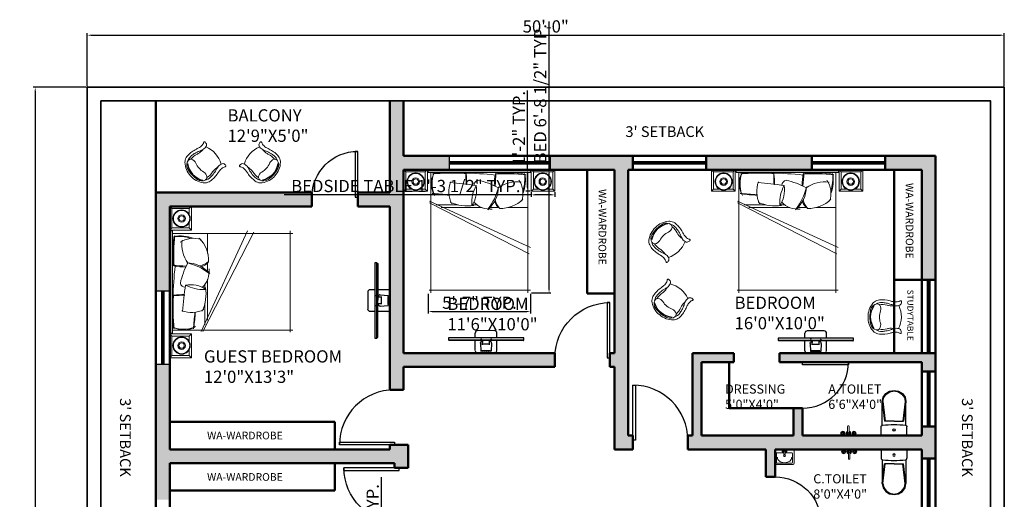
# Model space of a CAD drawing. Units: inches. Extents: x 2442 to 3851, y 589 to 2836.
# Tile 12 of 22: x 3165 to 3809, y 1732 to 2046. Entities that reach past the tile are written whole.
import ezdxf

# ---------------------------------------------------------------- set-up
doc = ezdxf.new("R2010")
doc.units = ezdxf.units.IN
for name, color, linetype, lineweight in [('0.10', 252, 'Continuous', 9), ('0.15', 34, 'Continuous', 15), ('A-ANNO-DIMS', 2, 'Continuous', 18), ('A-ANNO-TEXT', 7, 'Continuous', 18), ('A-AREA-IDEN', 7, 'Continuous', 18), ('A-DOOR', 4, 'Continuous', 25), ('A-FLOR-FIXT', 8, 'Continuous', 18), ('A-FURN', 8, 'Continuous', 18), ('A-GLAZ', 1, 'Continuous', 25), ('A-WALL', 7, 'Continuous', 50), ('A-WALL-PATT', 8, 'Continuous', 13), ('C-PROP', 7, 'Continuous', 35)]:
    doc.layers.add(name, color=color, linetype=linetype, lineweight=lineweight)
for name, color, linetype in [('IFF-FURN-DETAIL', 250, 'Continuous'), ('SANTEH', 7, 'Continuous'), ('window', 130, 'Continuous')]:
    doc.layers.add(name, color=color, linetype=linetype)
doc.styles.get("Standard").update_dxf_attribs({"font": 'arial.ttf'})
doc.dimstyles.new('ISO-25', dxfattribs={"dimtxt": 8, "dimasz": 2.5, "dimexe": 1.25, "dimexo": 0.625, "dimtad": 1, "dimlunit": 3, "dimtxsty": 'Standard', "dimcen": 2.5, "dimadec": 0, "dimazin": 0, "dimtfac": 1, "dimtmove": 0, "dimatfit": 3, "dimfxl": 1, "dimarcsym": 0})

# ---------------------------------------------------------------- blocks, each defined once
blk = doc.blocks.new('*U23')
for p, q in [((0, 0), (0, -6)), ((36, 0), (36, -6))]:
    blk.add_line(p, q)
blk.add_lwpolyline([(0, 0), (0, 36), (1.75, 36), (1.75, 0)], close=True)
blk.add_arc((0, 0), 36, 0, 90)
blk = doc.blocks.new('*U24')
for p, q in [((0, 0), (0, -6)), ((30, 0), (30, -6))]:
    blk.add_line(p, q)
blk.add_lwpolyline([(0, 0), (0, 30), (1.75, 30), (1.75, 0)], close=True)
blk.add_arc((0, 0), 30, 0, 90)
blk = doc.blocks.new('camita')
at = {"layer": '0.10'}
for p, q in [((-0.85, -0.045), (0.85, -0.045)), ((-0.805, -0.045), (-0.805, -2.048)), ((0.805, -0.045), (0.805, -2.048)), ((-0.827, -0.521), (0.846, -1.293)), ((-0.827, -0.548), (0.824, -1.399)), ((-0.716, -0.585), (-0.355, -0.585)), ((-0.638, -0.63), (0.043, -0.63)), ((-0.114, -0.585), (-0.049, -0.585)), ((0.175, -0.63), (0.318, -0.63)), ((0.474, -0.63), (0.805, -0.63)), ((-0.835, -2), (0.846, -2))]:
    blk.add_line(p, q, dxfattribs=at)
blk.add_lwpolyline([(-0.85, -0.041), (0.85, -0.041), (0.85, 0), (-0.85, 0)], close=True, dxfattribs=at)
for centre, radius, start, end in [((-0.457, -0.236), 0.344, 147.51, 213.8336), ((-0.2, -0.227), 0.586, 163.9263, 197.1409), ((-0.364, -5.846), 5.791, 83.8073, 94.1211), ((-0.51, -1.723), 1.678, 80.1255, 98.6619), ((2.353, -0.053), 2.58, 180.1063, 184.3854), ((-1.544, -0.245), 1.333, 359.9394, 7.5533), ((1.581, -0.289), 1.335, 170.3802, 178.9914), ((-1.44, -0.061), 1.712, 352.9291, 0.3959), ((0.452, -3.067), 3, 83.9026, 93.6759), ((0.486, -1.629), 1.578, 80.1602, 98.06), ((0.029, -0.138), 0.726, 342.5841, 6.0048), ((0.133, -0.17), 0.631, 339.923, 8.7433), ((-0.054, -0.363), 0.454, 159.3026, 206.5026), ((-1.33, -9.675), 9.499, 82.2708, 84.9399), ((0.458, -0.545), 0.584, 151.0456, 184.1497), ((-0.534, -0.339), 0.487, 327.2644, 9.0473), ((-0.007, -0.258), 0.0828, 100.018, 179.736), ((-0.293, -1.438), 1.29, 61.9749, 77.8435), ((-0.199, -0.274), 0.516, 310.7395, 359.0576), ((-0.567, -0.087), 0.906, 321.6953, 346.4626), ((0.627, -0.752), 0.551, 82.9691, 124.6739), ((0.32, -0.394), 0.404, 341.4524, 33.4512), ((-1.867, -14.986), 14.632, 84.6597, 85.7516), ((-0.46, 1.486), 1.909, 260.953, 268.6517), ((-0.2, 0.064), 0.667, 244.7809, 279.0606), ((0.179, -0.272), 0.383, 224.5284, 275.2229), ((0.438, -0.483), 0.19, 193.6849, 236.7035), ((0.571, -0.432), 0.315, 192.9388, 221.9636), ((0.361, -0.133), 0.51, 267.2589, 315.2997)]:
    blk.add_arc(centre, radius, start, end, dxfattribs=at)
blk = doc.blocks.new('VELADOR')
at = {"layer": '0.15'}
for p, q in [((-0.248, 0), (-0.203, -0.045)), ((0.248, 0), (0.202, -0.045)), ((-0.203, -0.405), (-0.248, -0.45)), ((0.248, -0.45), (0.202, -0.405))]:
    blk.add_line(p, q, dxfattribs=at)
blk.add_lwpolyline([(-0.248, 0), (-0.248, -0.45), (0.248, -0.45), (0.248, 0)], close=True, dxfattribs=at)
blk.add_lwpolyline([(0.092, -0.405), (0.202, -0.405), (0.202, -0.045), (-0.203, -0.045), (-0.203, -0.405), (-0.082, -0.405)], dxfattribs=at)
for radius in [0.18, 0.169, 0.0788, 0.0563]:
    blk.add_circle((0.005, -0.247), radius, dxfattribs=at)
blk = doc.blocks.new('ILNG95')
for points in [[(120, 308, -0.32971), (51, 384, -0.036099), (50, 422, -0.497733), (75, 439, -0.070621), (96, 429, 0.101868), (133, 414, 0.091794), (259, 412, 0.024114), (351, 433, -0.090294), (638, 458, -0.132412), (775, 407, -0.068618), (816, 368, -0.184346), (943, 0, 1.803905)], [(120, 308, 0.138132), (244, 313, 0.001085), (325, 339, -0.034227), (462, 375, -0.033255), (567, 387, -0.137428), (727, 350, -4.561553)], [(120, 308, 0.138132), (244, 313, 0.001085), (325, 339, -0.034227), (462, 375, -0.033255), (567, 387, -0.137428), (727, 350, -4.561553)], [(235, 308, 0.064243), (394, 307, 0.04414), (433, 315, -0.118032), (643, 329, -6.296816)], [(235, 308, 0.064243), (394, 307, 0.04414), (433, 315, -0.118032), (643, 329, -6.296816)], [(639, 0, 0.078302), (612, 161, -0.233633), (633, 315, -0.28763), (710, 349, -0.317923), (875, 193, -0.032882), (900, 0, 1.140397)], [(639, 0, 0.078302), (612, 161, -0.233633), (633, 315, -0.28763), (710, 349, -0.317923), (875, 193, -0.032882), (900, 0, 1.140397)], [(120, -308, 0.32971), (51, -384, 0.036099), (50, -422, 0.497733), (75, -439, 0.070621), (96, -429, -0.101868), (133, -414, -0.091794), (259, -412, -0.024114), (351, -433, 0.090294), (638, -458, 0.132412), (775, -407, 0.068618), (816, -368, 0.184346), (943, 0, -1.803905)], [(639, 0, -0.078302), (612, -161, 0.233633), (633, -315, 0.28763), (710, -349, 0.317923), (875, -193, 0.032882), (900, 0, -1.140397)], [(639, 0, -0.078302), (612, -161, 0.233633), (633, -315, 0.28763), (710, -349, 0.317923), (875, -193, 0.032882), (900, 0, -1.140397)], [(120, -308, -0.138132), (244, -313, -0.001085), (325, -339, 0.034227), (462, -375, 0.033255), (567, -387, 0.137428), (727, -350, 4.561553)], [(120, -308, -0.138132), (244, -313, -0.001085), (325, -339, 0.034227), (462, -375, 0.033255), (567, -387, 0.137428), (727, -350, 4.561553)], [(235, -308, -0.064243), (394, -307, -0.04414), (433, -315, 0.118032), (643, -329, 6.296816)], [(235, -308, -0.064243), (394, -307, -0.04414), (433, -315, 0.118032), (643, -329, 6.296816)]]:
    blk.add_lwpolyline(points, format="xyb")
blk.add_arc((759, 1), 709, 154.3281, 205.801)
at = {"layer": 'IFF-FURN-DETAIL'}
blk.add_arc((326, -2), 549, 326.8997, 34.6691, dxfattribs=at)
blk.add_arc((326, -2), 549, 326.8997, 34.6691, dxfattribs=at)
blk = doc.blocks.new('TV')
at = {"color": 0}
for p, q in [((3967.27, 1784.85), (3967.05, 1784.65)), ((3967.76, 1763.68), (3967.54, 1763.86))]:
    blk.add_line(p, q, dxfattribs=at)
at = {"layer": 'window'}
for p, q in [((3967.54, 1763.86), (3967.05, 1784.65)), ((3964.41, 1777.23), (3967.22, 1777.3)), ((3968.01, 1777.32), (3969.36, 1777.35)), ((3966.53, 1775.82), (3964.33, 1775.61)), ((3964.34, 1775.34), (3964.45, 1775.34)), ((3964.34, 1775.31), (3964.43, 1775.32)), ((3966.14, 1775.2), (3967.01, 1775.22)), ((3966.14, 1775.18), (3967.27, 1775.2)), ((3966.14, 1775.18), (3966.14, 1775.2)), ((3966.3, 1773.29), (3966.26, 1775.18)), ((3964.39, 1773.06), (3964.48, 1773.06)), ((3964.39, 1773.04), (3964.5, 1773.04)), ((3966.61, 1772.66), (3964.4, 1772.77)), ((3966.19, 1773.28), (3967.31, 1773.31)), ((3966.19, 1773.26), (3967.05, 1773.28)), ((3966.19, 1773.26), (3966.19, 1773.28)), ((3964.55, 1771.15), (3967.36, 1771.22)), ((3968.15, 1771.24), (3969.5, 1771.27))]:
    blk.add_line(p, q, dxfattribs=at)
for points in [[(3968.33, 1763.69), (3967.83, 1784.86), (3967.27, 1784.85), (3967.76, 1763.68), (3968.33, 1763.69)], [(3963.86, 1771.81), (3963.75, 1776.54)], [(3964.4, 1772.77), (3964.33, 1775.61)], [(3964.48, 1773.06), (3964.43, 1775.32)], [(3964.5, 1773.04), (3964.45, 1775.34)], [(3970.16, 1771.96), (3970.05, 1776.69)]]:
    blk.add_lwpolyline(points, dxfattribs=at)
for points in [[(3966.53, 1775.82, -0.263666), (3966.93, 1775.69), (3967, 1775.57), (3967.01, 1775.22)], [(3966.61, 1772.66, 0.263666), (3967, 1772.81), (3967.06, 1772.93), (3967.05, 1773.28)]]:
    blk.add_lwpolyline(points, format="xyb", dxfattribs=at)
for centre, radius in [((3963.91, 1775.73), 0.0679), ((3963.93, 1775.17), 0.0679), ((3963.94, 1774.6), 0.0679), ((3967.77, 1775.68), 0.0451), ((3963.95, 1774.04), 0.0679), ((3963.97, 1773.48), 0.0679), ((3963.98, 1772.92), 0.0679), ((3963.99, 1772.35), 0.0679), ((3964.01, 1771.79), 0.0679), ((3967.83, 1772.86), 0.0451)]:
    blk.add_circle(centre, radius, dxfattribs=at)
for centre, start, end in [((3964.42, 1776.56), 91.3414, 181.3414), ((3969.38, 1776.67), 1.3414, 91.3414), ((3964.53, 1771.83), 181.3414, 271.3414), ((3969.49, 1771.94), 271.3414, 1.3414)]:
    blk.add_arc(centre, 0.676, start, end, dxfattribs=at)
blk = doc.blocks.new('WC 2 Symb_109')
at = {"layer": 'SANTEH'}
for p, q in [((0, 0), (0, 380)), ((0, 380), (132, 380)), ((154, 365), (507, 365)), ((506, 365), (216, 331)), ((506, 356), (216, 322)), ((216, 190), (216, 331)), ((216, 190), (216, 49)), ((154, 15), (507, 15)), ((506, 24), (216, 58)), ((506, 15), (216, 49)), ((0, 0), (132, 0))]:
    blk.add_line(p, q, dxfattribs=at)
for points in [[(155, 360), (154, 364), (152, 368), (150, 371), (147, 374), (144, 377), (140, 379), (137, 380), (132, 380)], [(155, 20), (159, 62), (161, 105), (163, 147), (164, 190), (163, 233), (161, 275), (159, 318), (155, 360)], [(506, 24), (565, 37), (616, 73), (649, 126), (661, 190), (649, 254), (616, 307), (565, 343), (506, 356)], [(507, 15), (569, 28), (622, 66), (658, 123), (670, 190), (658, 257), (622, 314), (569, 352), (507, 365)], [(132, 0), (136, 0), (140, 1), (144, 3), (147, 6), (150, 9), (152, 12), (154, 16), (155, 20)]]:
    blk.add_lwpolyline(points, dxfattribs=at)
blk.add_lwpolyline([(84, 208), (70, 203), (65, 190), (70, 177), (84, 172), (97, 177), (102, 190), (97, 203)], close=True, dxfattribs=at)
blk = doc.blocks.new('Faucet - Bathroom top')
for p, q in [((-4.107, 0.125), (-4.375, 0.125)), ((-3.75, 0.4788), (-3.75, 0.75)), ((-3.5, 0.482), (-3.5, 0.75)), ((-3.1461, 0.125), (-2.875, 0.125)), ((3.143, 0.125), (2.875, 0.125)), ((3.5, 0.4788), (3.5, 0.75)), ((3.75, 0.482), (3.75, 0.75)), ((4.1039, 0.125), (4.375, 0.125)), ((-4.1039, -0.125), (-4.375, -0.125)), ((-3.75, -0.4821), (-3.75, -0.75)), ((-3.5, -0.4789), (-3.5, -0.75)), ((-3.143, -0.125), (-2.875, -0.125)), ((-0.5, -0.8639), (-0.5, -4.5)), ((0.5, -4.5), (0.5, -0.8631)), ((3.1461, -0.125), (2.875, -0.125)), ((3.5, -0.4821), (3.5, -0.75)), ((3.75, -0.4789), (3.75, -0.75)), ((4.107, -0.125), (4.375, -0.125))]:
    blk.add_line(p, q)
for centre, radius in [((-3.625, 0), 1.375), ((-4.625, 0), 0.2795), ((-3.625, 0), 0.5), ((-3.625, 1), 0.2795), ((-2.625, 0), 0.2795), ((0, 0), 0.5), ((3.625, 0), 1.375), ((2.625, 0), 0.2795), ((3.625, 0), 0.5), ((3.625, 1), 0.2795), ((4.625, 0), 0.2795), ((-3.625, -1), 0.2795), ((3.625, -1), 0.2795)]:
    blk.add_circle(centre, radius)
for centre, radius, start, end in [((-3.625, 0), 1, 105.2407, 164.2093), ((-3.625, 0), 1, 16.44125, 74.07887), ((0, 0), 1.5, 289.6514, 250.3603), ((0, 0), 1, 300.3431, 239.7554), ((3.625, 0), 1, 106.12, 164.0884), ((3.625, 0), 1, 16.23422, 73.90469), ((-3.625, 0), 1, 196.2342, 253.9047), ((-3.625, 0), 1, 286.12, 344.0884), ((0, -4.5), 0.5, 180, 0), ((3.625, 0), 1, 196.4413, 254.0789), ((3.625, 0), 1, 285.2407, 344.2093)]:
    blk.add_arc(centre, radius, start, end)
blk = doc.blocks.new('Rac7')
at = {"color": 0}
for p, q in [((-39501, -24232), (-39501, -23830)), ((-39474, -23808), (-38988, -23808)), ((-39457, -23859), (-39457, -24115)), ((-39032, -23838), (-39430, -23838)), ((-39221, -23855), (-39241, -23855)), ((-39005, -24115), (-39005, -23859)), ((-39005, -23859), (-39005, -23859)), ((-38961, -23830), (-38961, -24232)), ((-38961, -24232), (-39501, -24232)), ((-39430, -24136), (-39253, -24136)), ((-39297, -24164), (-39253, -24164)), ((-39297, -24194), (-39297, -24164)), ((-39165, -24194), (-39297, -24194)), ((-39253, -24186), (-39253, -24094)), ((-39253, -24186), (-39209, -24186)), ((-39209, -24186), (-39209, -24094)), ((-39209, -24136), (-39032, -24136)), ((-39209, -24164), (-39165, -24164)), ((-39165, -24164), (-39165, -24194))]:
    blk.add_line(p, q, dxfattribs=at)
at = {"color": 0, "extrusion": (0, 0, -1)}
for centre, major_axis, start_param, end_param in [((-39474, -23830), (-27, 0), 0, 1.570796), ((-39430, -23859), (-27, 0), 0, 1.570796), ((-39241, -24007), (-194, 0), 0, 1.570796), ((-39221, -24007), (-194, 0), 1.570796, 3.141593), ((-39032, -23859), (-27, 0), 1.570796, 3.141593), ((-38988, -23830), (-27, 0), 1.570796, 3.141593), ((-39430, -24115), (-27, 0), -1.570796, 0), ((-39231, -24104), (-25.3, 0), 0.552816, 2.588777), ((-39032, -24115), (-27, 0), -3.141593, -1.570796)]:
    blk.add_ellipse(centre, major_axis=major_axis, ratio=0.785714, start_param=start_param, end_param=end_param, dxfattribs=at)
blk.add_ellipse((-39231, -24048), major_axis=(-27.9, 0), ratio=0.785714, dxfattribs=at)
blk = doc.blocks.new('*D140')
at = {"layer": 'A-ANNO-DIMS', "color": 0, "lineweight": -2, "transparency": 16777216}
for p, q in [((3510.97, 1947.86), (3510.97, 2044.75)), ((3499.5, 1947.86), (3512.22, 1947.86)), ((3510.97, 1869.71), (3510.97, 1945.36)), ((3499.5, 1867.21), (3512.22, 1867.21))]:
    blk.add_line(p, q, dxfattribs=at)
at = {"layer": 'A-ANNO-DIMS', "color": 0, "transparency": 16777216}
for points in [[(3510.55, 1945.36), (3511.39, 1945.36), (3510.97, 1947.86)], [(3510.55, 1869.71), (3511.39, 1869.71), (3510.97, 1867.21)]]:
    blk.add_solid(points, dxfattribs=at)
at = {"layer": 'Defpoints', "color": 0, "transparency": 16777216}
for p in [(3498.87, 1947.86), (3510.97, 1947.86), (3498.87, 1867.21)]:
    blk.add_point(p, dxfattribs=at)
at = {"layer": 'A-ANNO-DIMS', "color": 0, "transparency": 16777216, "insert": (3506.21, 1997.56), "char_height": 8, "attachment_point": 5, "rotation": 90}
blk.add_mtext('BED 6\'-8 1/2" TYP.', dxfattribs=at)
blk = doc.blocks.new('*D141')
at = {"layer": 'A-ANNO-DIMS', "color": 0, "lineweight": -2, "transparency": 16777216}
for p, q in [((3431.94, 1866.58), (3431.94, 1853.86)), ((3498.87, 1866.58), (3498.87, 1853.86)), ((3434.44, 1855.11), (3496.37, 1855.11))]:
    blk.add_line(p, q, dxfattribs=at)
at = {"layer": 'A-ANNO-DIMS', "color": 0, "transparency": 16777216}
for points in [[(3434.44, 1855.52), (3434.44, 1854.69), (3431.94, 1855.11)], [(3496.37, 1855.52), (3496.37, 1854.69), (3498.87, 1855.11)]]:
    blk.add_solid(points, dxfattribs=at)
at = {"layer": 'Defpoints', "color": 0, "transparency": 16777216}
for p in [(3431.94, 1867.21), (3498.87, 1867.21), (3498.87, 1855.11)]:
    blk.add_point(p, dxfattribs=at)
at = {"layer": 'A-ANNO-DIMS', "color": 0, "transparency": 16777216, "insert": (3465.4, 1859.8), "char_height": 8, "attachment_point": 5}
blk.add_mtext('5\'-7" TYP.', dxfattribs=at)
blk = doc.blocks.new('*D142')
at = {"layer": 'A-ANNO-DIMS', "color": 0, "lineweight": -2, "transparency": 16777216}
for p, q in [((3499.25, 1933.1), (3499.25, 1930.14)), ((3514.8, 1933.1), (3514.8, 1930.14)), ((3499.25, 1931.39), (3337.77, 1931.39)), ((3512.3, 1931.39), (3501.75, 1931.39))]:
    blk.add_line(p, q, dxfattribs=at)
at = {"layer": 'A-ANNO-DIMS', "color": 0, "transparency": 16777216}
for points in [[(3501.75, 1931.81), (3501.75, 1930.98), (3499.25, 1931.39)], [(3512.3, 1931.81), (3512.3, 1930.98), (3514.8, 1931.39)]]:
    blk.add_solid(points, dxfattribs=at)
at = {"layer": 'Defpoints', "color": 0, "transparency": 16777216}
for p in [(3499.25, 1933.73), (3514.8, 1933.73), (3499.25, 1931.39)]:
    blk.add_point(p, dxfattribs=at)
at = {"layer": 'A-ANNO-DIMS', "color": 0, "transparency": 16777216, "insert": (3417.26, 1936.16), "char_height": 8, "attachment_point": 5}
blk.add_mtext('BEDSIDE TABLE 1\'-3 1/2" TYP.', dxfattribs=at)
blk = doc.blocks.new('*D143')
at = {"layer": 'A-ANNO-DIMS', "color": 0, "lineweight": -2, "transparency": 16777216}
for p, q in [((3496.91, 1947.86), (3496.91, 1999.62)), ((3498.62, 1947.86), (3495.66, 1947.86)), ((3496.91, 1936.23), (3496.91, 1945.36)), ((3498.62, 1933.73), (3495.66, 1933.73))]:
    blk.add_line(p, q, dxfattribs=at)
at = {"layer": 'A-ANNO-DIMS', "color": 0, "transparency": 16777216}
for points in [[(3496.5, 1945.36), (3497.33, 1945.36), (3496.91, 1947.86)], [(3496.5, 1936.23), (3497.33, 1936.23), (3496.91, 1933.73)]]:
    blk.add_solid(points, dxfattribs=at)
at = {"layer": 'Defpoints', "color": 0, "transparency": 16777216}
for p in [(3496.91, 1947.86), (3499.25, 1947.86), (3499.25, 1933.73)]:
    blk.add_point(p, dxfattribs=at)
at = {"layer": 'A-ANNO-DIMS', "color": 0, "transparency": 16777216, "insert": (3492.27, 1974.99), "char_height": 8, "attachment_point": 5, "rotation": 90}
blk.add_mtext('1\'-2" TYP.', dxfattribs=at)
blk = doc.blocks.new('*D172')
at = {"layer": 'A-ANNO-DIMS', "color": 0, "lineweight": -2, "transparency": 16777216}
for p, q in [((3401.36, 1596.65), (3401.36, 1746.62)), ((3396.93, 1596.65), (3402.61, 1596.65)), ((3401.36, 1565.43), (3401.36, 1594.15)), ((3396.93, 1562.93), (3402.61, 1562.93))]:
    blk.add_line(p, q, dxfattribs=at)
at = {"layer": 'A-ANNO-DIMS', "color": 0, "transparency": 16777216}
for points in [[(3400.94, 1594.15), (3401.78, 1594.15), (3401.36, 1596.65)], [(3400.94, 1565.43), (3401.78, 1565.43), (3401.36, 1562.93)]]:
    blk.add_solid(points, dxfattribs=at)
at = {"layer": 'Defpoints', "color": 0, "transparency": 16777216}
for p in [(3396.3, 1596.65), (3401.36, 1596.65), (3396.3, 1562.93)]:
    blk.add_point(p, dxfattribs=at)
at = {"layer": 'A-ANNO-DIMS', "color": 0, "transparency": 16777216, "insert": (3396.6, 1672.89), "char_height": 8, "attachment_point": 5, "rotation": 90}
blk.add_mtext('STUDY CHAIR 2\'-9 1/2" TYP.', dxfattribs=at)
blk = doc.blocks.new('*D256')
at = {"layer": 'A-ANNO-DIMS', "color": 0, "lineweight": -2, "transparency": 16777216}
for p, q in [((3208.8, 2002.49), (3208.8, 2037.11)), ((3211.3, 2035.86), (3806.3, 2035.86)), ((3808.8, 2002.49), (3808.8, 2037.11))]:
    blk.add_line(p, q, dxfattribs=at)
at = {"layer": 'A-ANNO-DIMS', "color": 0, "transparency": 16777216}
for points in [[(3211.3, 2036.28), (3211.3, 2035.45), (3208.8, 2035.86)], [(3806.3, 2036.28), (3806.3, 2035.45), (3808.8, 2035.86)]]:
    blk.add_solid(points, dxfattribs=at)
at = {"layer": 'Defpoints', "color": 0, "transparency": 16777216}
for p in [(3808.8, 2035.86), (3208.8, 2001.86), (3808.8, 2001.86)]:
    blk.add_point(p, dxfattribs=at)
at = {"layer": 'A-ANNO-DIMS', "color": 0, "transparency": 16777216, "insert": (3508.8, 2040.57), "char_height": 8, "attachment_point": 5}
blk.add_mtext('50\'-0"', dxfattribs=at)
blk = doc.blocks.new('*D257')
at = {"layer": 'A-ANNO-DIMS', "color": 0, "lineweight": -2, "transparency": 16777216}
for p, q in [((3208.17, 2001.86), (3173.55, 2001.86)), ((3174.8, 1999.36), (3174.8, 1404.36)), ((3208.17, 1401.86), (3173.55, 1401.86))]:
    blk.add_line(p, q, dxfattribs=at)
at = {"layer": 'A-ANNO-DIMS', "color": 0, "transparency": 16777216}
for points in [[(3174.38, 1999.36), (3175.21, 1999.36), (3174.8, 2001.86)], [(3174.38, 1404.36), (3175.21, 1404.36), (3174.8, 1401.86)]]:
    blk.add_solid(points, dxfattribs=at)
at = {"layer": 'Defpoints', "color": 0, "transparency": 16777216}
for p in [(3208.8, 2001.86), (3174.8, 1401.86), (3208.8, 1401.86)]:
    blk.add_point(p, dxfattribs=at)
at = {"layer": 'A-ANNO-DIMS', "color": 0, "transparency": 16777216, "insert": (3170.09, 1701.86), "char_height": 8, "attachment_point": 5, "rotation": 90}
blk.add_mtext('50\'-0"', dxfattribs=at)

msp = doc.modelspace()

# ---------------------------------------------------------------- hatches: boundary and pattern name
at = {"layer": 'A-WALL-PATT'}
h = msp.add_hatch(color=256, dxfattribs=at)
h.dxf.hatch_style = 1
h.paths.add_polyline_path([(3262.798, 1497.864), (3268.798, 1497.864), (3268.798, 1503.864), (3268.798, 1506.864), (3262.798, 1506.864), (3262.798, 1530.864), (3253.798, 1530.864), (3253.798, 1401.864), (3262.798, 1401.864)])
h.paths.add_polyline_path([(3418.798, 1506.864), (3385.798, 1506.864), (3385.798, 1497.864), (3409.798, 1497.864), (3409.798, 1401.864), (3418.798, 1401.864), (3418.798, 1458.864), (3448.798, 1458.864), (3448.798, 1467.864), (3424.616, 1467.864), (3418.798, 1467.864)])
h.paths.add_polyline_path([(3319.798, 1506.864), (3308.798, 1506.864), (3308.798, 1497.864), (3319.798, 1497.864)])
h.paths.add_polyline_path([(3514.798, 1467.864), (3490.798, 1467.864), (3490.798, 1458.864), (3514.798, 1458.864)])
h.paths.add_polyline_path([(3607.798, 1497.864), (3598.798, 1497.864), (3598.798, 1488.228), (3598.798, 1467.864), (3580.798, 1467.864), (3580.798, 1458.864), (3607.798, 1458.864)])
h.paths.add_polyline_path([(3418.798, 1716.864), (3409.798, 1716.864), (3409.798, 1611.864), (3262.798, 1611.864), (3262.798, 1683.864), (3253.798, 1683.864), (3253.798, 1578.864), (3262.798, 1578.864), (3262.798, 1602.864), (3409.798, 1602.864), (3409.798, 1554.864), (3418.798, 1554.864)])
h.paths.add_polyline_path([(3418.798, 1767.864), (3406.798, 1767.864), (3406.798, 1764.864), (3262.798, 1764.864), (3262.798, 1820.364), (3253.798, 1820.364), (3253.798, 1731.864), (3262.798, 1731.864), (3262.798, 1755.864), (3409.798, 1755.864), (3409.798, 1752.864), (3412.798, 1752.864), (3418.798, 1752.864)])
h.paths.add_polyline_path([(3355.798, 1932.864), (3253.798, 1932.864), (3253.798, 1868.364), (3262.798, 1868.364), (3262.798, 1907.939), (3262.798, 1923.864), (3276.934, 1923.864), (3355.798, 1923.864), (3355.798, 1929.864)])
h.paths.add_polyline_path([(3415.798, 1992.864), (3406.798, 1992.864), (3406.798, 1932.864), (3385.798, 1932.864), (3385.798, 1923.864), (3406.798, 1923.864), (3406.798, 1803.864), (3415.798, 1803.864), (3415.798, 1818.864), (3514.798, 1818.864), (3514.798, 1827.864), (3415.798, 1827.864), (3415.798, 1947.864), (3445.798, 1947.864), (3445.798, 1956.864), (3415.798, 1956.864)])
h.paths.add_polyline_path([(3565.798, 1956.864), (3511.798, 1956.864), (3511.798, 1947.864), (3514.798, 1947.864), (3553.798, 1947.864), (3553.798, 1827.864), (3550.798, 1827.864), (3550.798, 1824.864), (3550.798, 1818.864), (3553.798, 1818.864), (3553.798, 1764.864), (3565.798, 1764.864), (3565.798, 1770.864), (3565.798, 1773.864), (3562.798, 1773.864), (3562.798, 1947.864), (3565.798, 1947.864)])
h.paths.add_polyline_path([(3682.798, 1956.864), (3613.798, 1956.864), (3613.798, 1947.864), (3682.798, 1947.864)])
h.paths.add_polyline_path([(3763.798, 1956.864), (3730.798, 1956.864), (3730.798, 1947.864), (3754.798, 1947.864), (3754.798, 1875.864), (3763.798, 1875.864)])
h.paths.add_polyline_path([(3763.798, 1827.864), (3661.798, 1827.864), (3661.798, 1821.864), (3754.798, 1821.864), (3754.798, 1815.864), (3763.798, 1815.864)])
h.paths.add_polyline_path([(3763.798, 1779.864), (3754.798, 1779.864), (3754.798, 1773.864), (3707.032, 1773.864, -0.0790467), (3706.561, 1773.864), (3676.798, 1773.864), (3676.798, 1791.864), (3670.798, 1791.864), (3670.798, 1773.864), (3610.798, 1773.864), (3610.798, 1821.864), (3631.798, 1821.864), (3631.798, 1827.864), (3604.798, 1827.864), (3604.798, 1773.864), (3601.798, 1773.864), (3601.798, 1764.864), (3652.798, 1764.864), (3652.798, 1746.864), (3658.798, 1746.864), (3658.798, 1764.864), (3671.259, 1764.864), (3754.798, 1764.864), (3754.798, 1758.864), (3763.798, 1758.864)])
h.paths.add_polyline_path([(3763.798, 1722.864), (3754.798, 1722.864), (3754.798, 1716.864), (3652.798, 1716.864), (3652.798, 1710.864), (3754.798, 1710.864), (3754.798, 1685.364), (3763.798, 1685.364)])
h.paths.add_polyline_path([(3607.798, 1671.864), (3598.798, 1671.864), (3598.798, 1563.864), (3607.798, 1563.864), (3607.798, 1602.864), (3763.798, 1602.864), (3763.798, 1637.364), (3754.798, 1637.364), (3754.798, 1611.864), (3607.798, 1611.864)])

# ---------------------------------------------------------------- linework, layer by layer
at = {"layer": 'A-GLAZ'}
for p, q in [((3445.798, 1947.864), (3445.798, 1956.864)), ((3511.798, 1947.864), (3511.798, 1956.864)), ((3262.798, 1868.364), (3253.798, 1868.364)), ((3262.798, 1820.364), (3253.798, 1820.364))]:
    msp.add_line(p, q, dxfattribs=at)
at = {"layer": 'A-WALL'}
for p, q in [((3253.798, 1992.864), (3253.798, 1401.864)), ((3406.798, 1932.864), (3406.798, 1992.864)), ((3415.798, 1956.864), (3415.798, 1992.864)), ((3415.798, 1956.864), (3763.798, 1956.864)), ((3445.798, 1952.864), (3511.798, 1952.864)), ((3445.798, 1951.864), (3511.798, 1951.864)), ((3565.798, 1947.864), (3565.798, 1956.864)), ((3565.798, 1952.864), (3613.798, 1952.864)), ((3565.798, 1951.864), (3613.798, 1951.864)), ((3613.798, 1947.864), (3613.798, 1956.864)), ((3682.798, 1947.864), (3682.798, 1956.864)), ((3682.798, 1952.864), (3730.798, 1952.864)), ((3682.798, 1951.864), (3730.798, 1951.864)), ((3730.798, 1947.864), (3730.798, 1956.864)), ((3763.798, 1602.864), (3763.798, 1956.864)), ((3415.798, 1947.864), (3553.798, 1947.864)), ((3415.798, 1827.864), (3415.798, 1947.864)), ((3535.798, 1866.864), (3535.798, 1947.864)), ((3553.798, 1827.864), (3553.798, 1947.864)), ((3562.798, 1773.864), (3562.798, 1947.864)), ((3562.798, 1947.864), (3754.798, 1947.864)), ((3736.798, 1827.864), (3736.798, 1947.864)), ((3754.798, 1827.864), (3754.798, 1947.864)), ((3253.798, 1932.864), (3355.798, 1932.864)), ((3355.798, 1923.864), (3355.798, 1932.864)), ((3385.798, 1923.864), (3385.798, 1932.864)), ((3385.798, 1932.864), (3406.798, 1932.864)), ((3262.798, 1923.864), (3262.798, 1764.864)), ((3262.798, 1923.864), (3355.798, 1923.864)), ((3385.798, 1923.864), (3406.798, 1923.864)), ((3406.798, 1803.864), (3406.798, 1923.864)), ((3736.798, 1875.864), (3763.798, 1875.864)), ((3758.798, 1827.864), (3758.798, 1875.864)), ((3759.798, 1827.864), (3759.798, 1875.864)), ((3257.798, 1868.364), (3257.798, 1820.364)), ((3258.798, 1868.364), (3258.798, 1820.364)), ((3535.798, 1866.864), (3553.798, 1866.864)), ((3415.798, 1827.864), (3514.798, 1827.864)), ((3514.798, 1818.864), (3514.798, 1827.864)), ((3550.798, 1818.864), (3550.798, 1827.864)), ((3550.798, 1827.864), (3553.798, 1827.864)), ((3604.798, 1773.864), (3604.798, 1827.864)), ((3604.798, 1827.864), (3631.798, 1827.864)), ((3631.798, 1821.864), (3631.798, 1827.864)), ((3661.798, 1821.864), (3661.798, 1827.864)), ((3661.798, 1827.864), (3763.798, 1827.864)), ((3415.798, 1818.864), (3514.798, 1818.864)), ((3415.798, 1803.864), (3415.798, 1818.864)), ((3550.798, 1818.864), (3553.798, 1818.864)), ((3553.798, 1764.864), (3553.798, 1818.864)), ((3610.798, 1773.864), (3610.798, 1821.864)), ((3610.798, 1821.864), (3631.798, 1821.864)), ((3628.798, 1791.864), (3628.798, 1821.864)), ((3661.798, 1821.864), (3754.798, 1821.864)), ((3754.798, 1773.864), (3754.798, 1821.864)), ((3754.798, 1815.864), (3763.798, 1815.864)), ((3758.798, 1779.864), (3758.798, 1815.864)), ((3759.798, 1779.864), (3759.798, 1815.864)), ((3406.798, 1803.864), (3415.798, 1803.864)), ((3628.798, 1791.864), (3670.798, 1791.864)), ((3670.798, 1773.864), (3670.798, 1791.864)), ((3670.798, 1791.864), (3676.798, 1791.864)), ((3676.798, 1773.864), (3676.798, 1791.864)), ((3262.798, 1782.864), (3370.798, 1782.864)), ((3370.798, 1764.864), (3370.798, 1782.864)), ((3754.798, 1779.864), (3763.798, 1779.864)), ((3562.798, 1773.864), (3565.798, 1773.864)), ((3565.798, 1764.864), (3565.798, 1773.864)), ((3601.798, 1764.864), (3601.798, 1773.864)), ((3601.798, 1773.864), (3604.798, 1773.864)), ((3610.798, 1773.864), (3670.798, 1773.864)), ((3676.798, 1773.864), (3754.798, 1773.864)), ((3406.798, 1764.864), (3406.798, 1767.864)), ((3406.798, 1767.864), (3418.798, 1767.864)), ((3418.798, 1752.864), (3418.798, 1767.864)), ((3262.798, 1764.864), (3406.798, 1764.864)), ((3553.798, 1764.864), (3565.798, 1764.864)), ((3601.798, 1764.864), (3652.798, 1764.864)), ((3652.798, 1746.864), (3652.798, 1764.864)), ((3658.798, 1746.864), (3658.798, 1764.864)), ((3658.798, 1764.864), (3754.798, 1764.864)), ((3754.798, 1716.864), (3754.798, 1764.864)), ((3754.798, 1758.864), (3763.798, 1758.864)), ((3758.798, 1722.864), (3758.798, 1758.864)), ((3759.798, 1722.864), (3759.798, 1758.864)), ((3262.798, 1755.864), (3262.798, 1611.864)), ((3262.798, 1755.864), (3409.798, 1755.864)), ((3370.798, 1755.864), (3370.798, 1737.864)), ((3409.798, 1752.864), (3409.798, 1755.864)), ((3409.798, 1752.864), (3418.798, 1752.864)), ((3652.798, 1746.864), (3658.798, 1746.864)), ((3262.798, 1737.864), (3370.798, 1737.864))]:
    msp.add_line(p, q, dxfattribs=at)
at = {"layer": 'C-PROP'}
for points in [[(3808.798, 1401.864), (3808.798, 2001.864), (3208.798, 2001.864), (3208.798, 1401.864), (3808.798, 1401.864)], [(3799.798, 1410.864), (3799.798, 1992.864), (3217.798, 1992.864), (3217.798, 1410.864), (3253.798, 1410.864)]]:
    msp.add_lwpolyline(points, dxfattribs=at)

# ---------------------------------------------------------------- block references
at = {"layer": 'A-DOOR', "xscale": -1}
for name, p in [('*U24', (3385.798, 1929.864)), ('*U23', (3550.798, 1824.864))]:
    msp.add_blockref(name, p, dxfattribs=at)
at = {"layer": 'A-DOOR'}
for name, p, rotation in [('*U24', (3676.798, 1821.864), 269.9999999999969), ('*U23', (3409.798, 1767.864), 90.00000000000003)]:
    msp.add_blockref(name, p, dxfattribs=dict(at, rotation=rotation))
msp.add_blockref('*U23', (3565.798, 1770.864), dxfattribs=at)
at = {"layer": 'A-DOOR', "xscale": -1}
for name, p, rotation in [('*U23', (3412.798, 1752.864), 90), ('*U24', (3658.798, 1716.864), 270)]:
    msp.add_blockref(name, p, dxfattribs=dict(at, rotation=rotation))
at = {"layer": 'A-FLOR-FIXT'}
for name, p, xscale, yscale, zscale, rotation in [('WC 2 Symb_109', (3728.281, 1773.864), -0.0441898926459964, 0.0441898926459964, 0.0441898926459964, 270.0000000000001), ('Rac7', (2758.42, 1204.872), 0.0231094998546128, 0.0231094998546128, 0.0231094998546128, 179.9999999999958), ('WC 2 Symb_109', (3728.281, 1764.864), 0.0441898926459964, 0.0441898926459964, 0.0441898926459964, 269.9999999999999)]:
    msp.add_blockref(name, p, dxfattribs=dict(at, xscale=xscale, yscale=yscale, zscale=zscale, rotation=rotation))
at = {"layer": 'A-FLOR-FIXT', "xscale": -1, "rotation": 180}
msp.add_blockref('Faucet - Bathroom top', (3706.797, 1775.345), dxfattribs=at)
at = {"layer": 'A-FLOR-FIXT'}
msp.add_blockref('Faucet - Bathroom top', (3707.3, 1763.364), dxfattribs=at)
at = {"layer": 'A-FURN'}
for name, p, xscale, yscale, zscale, rotation in [('ILNG95', (3293.626, 1959.125), 0.0243705291132055, 0.0243705291132055, 0.0243705291132055, 221.4118781376284), ('ILNG95', (3314.384, 1959.125), -0.0243705291132055, 0.0243705291132055, 0.0243705291132055, 138.5881218623715), ('VELADOR', (3507.022, 1947.864), -31.41542173157097, 31.41542173157097, 31.41542173157097, 359.9999999999999), ('VELADOR', (3708.469, 1947.864), -31.41542173157097, 31.41542173157097, 31.41542173157097, 359.9999999999999), ('VELADOR', (3262.798, 1916.089), -31.41542173157097, 31.41542173157097, 31.41542173157097, 89.99999999999991), ('ILNG95', (3596.544, 1893.529), 0.0243705291132055, 0.0243705291132055, 0.0243705291132055, 133.7094105413398), ('camita', (3262.798, 1874.471), 39.375, 39.375, 39.375, 90), ('TV', (12734.013, 5755.426), 2.327319231123021, 2.327319231123021, 2.327319231123021, 178.5430845181613), ('ILNG95', (3597.837, 1870.651), -0.0243705291132055, 0.0243705291132055, 0.0243705291132055, 50.88565426608293), ('ILNG95', (3742.663, 1851.412), -0.0243705291132055, 0.0243705291132055, 0.0243705291132055, 359.6824344718516), ('TV', (7362.902, -7499.166), 2.327319231123021, 2.327319231123021, 2.327319231123021, 88.54308451816127), ('TV', (7578.588, -7499.355), 2.327319231123021, 2.327319231123021, 2.327319231123021, 88.54308451816127), ('VELADOR', (3262.798, 1832.639), 31.41542173157097, 31.41542173157097, 31.41542173157097, 90)]:
    msp.add_blockref(name, p, dxfattribs=dict(at, xscale=xscale, yscale=yscale, zscale=zscale, rotation=rotation))
for name, p, xscale, yscale, zscale in [('VELADOR', (3423.573, 1947.864), 31.41542173157097, 31.41542173157097, 31.41542173157097), ('camita', (3465.404, 1947.864), 39.375, 39.375, 39.375), ('VELADOR', (3625.019, 1947.864), 31.41542173157097, 31.41542173157097, 31.41542173157097), ('camita', (3666.851, 1947.864), 39.375, 39.375, 39.375)]:
    msp.add_blockref(name, p, dxfattribs=dict(at, xscale=xscale, yscale=yscale, zscale=zscale))

# ---------------------------------------------------------------- texts
at = {"layer": 'A-ANNO-TEXT'}
for s, width, insert, char_height, attachment_point in [("{\\fTimes New Roman|b0|i0|c0|p18;3' SETBACK}", 79.56037, (3560.912, 1976.271), 7, 1), ('{\\fTimes New Roman|b0|i0|c0|p18;WA-WARDROBE}', 110.76054, (3287.245, 1771.428), 5, 7), ('{\\fTimes New Roman|b0|i0|c0|p18;WA-WARDROBE}', 110.76054, (3287.245, 1749.3), 5, 1)]:
    msp.add_mtext_dynamic_manual_height_columns(s, width=width, gutter_width=12.5, heights=[0], dxfattribs=dict(at, insert=insert, char_height=char_height, attachment_point=attachment_point))
at = {"layer": 'A-ANNO-TEXT', "attachment_point": 1, "rotation": 270}
for s, width, heights, insert, char_height in [('{\\fTimes New Roman|b0|i0|c0|p18;WA-WARDROBE}', 110.76054, [0], (3749.343, 1939.175), 5), ('{\\fTimes New Roman|b0|i0|c0|p18;WA-WARDROBE}', 110.76054, [0], (3548.343, 1935.167), 5), ('{\\fTimes New Roman|b0|i0|c0|p18;STUDYTABLE}', 110.76054, [5.476], (3749.343, 1869.361), 4), ("{\\fTimes New Roman|b0|i0|c0|p18;3' SETBACK}", 79.56037, [0], (3237.254, 1798.403), 7), ("{\\fTimes New Roman|b0|i0|c0|p18;3' SETBACK}", 79.56037, [0], (3788.094, 1798.403), 7)]:
    msp.add_mtext_dynamic_manual_height_columns(s, width=width, gutter_width=12.5, heights=heights, dxfattribs=dict(at, insert=insert, char_height=char_height))
at = {"layer": 'A-AREA-IDEN', "attachment_point": 1}
for s, insert, char_height in [('{\\fTimes New Roman|b0|i0|c0|p18;BALCONY\\P12\'9"X5\'0"}', (3300.603, 1987.409), 8), ('{\\fTimes New Roman|b0|i0|c0|p18;BEDROOM\\P11\'6"X10\'0"}', (3444.441, 1864.076), 8), ('{\\fTimes New Roman|b0|i0|c0|p18;BEDROOM\\P16\'0"X10\'0"}', (3632.353, 1864.776), 8), ('{\\fTimes New Roman|b0|i0|c0|p18;GUEST BEDROOM\\P12\'0"X13\'3"}', (3285.164, 1829.686), 8), ('{\\fTimes New Roman|b0|i0|c0|p18;DRESSING\\P5\'0"X4\'0"}', (3626.15, 1807.325), 6), ('{\\fTimes New Roman|b0|i0|c0|p18;A.TOILET\\P6\'6"X4\'0"}', (3693.636, 1807.325), 6), ('{\\fTimes New Roman|b0|i0|c0|p18;C.TOILET\\P8\'0"X4\'0"}', (3683.811, 1748.618), 6)]:
    msp.add_mtext_dynamic_manual_height_columns(s, width=110.76054, gutter_width=12.5, heights=[0], dxfattribs=dict(at, insert=insert, char_height=char_height))

# ---------------------------------------------------------------- dimensions: what is measured, and where the dimension line sits
at = {"layer": 'A-ANNO-DIMS'}
dim = msp.add_linear_dim(base=(3808.798, 2035.864), p1=(3208.798, 2001.864), p2=(3808.798, 2001.864), dimstyle='ISO-25', override={"dimdec": 1, "dimlfac": 1, "dimrnd": 0, "dimzin": 1, "dimdsep": 46, "dimlunit": 4, "dimfrac": 2}, dxfattribs=at)
dim.commit()
dim.dimension.update_dxf_attribs({"geometry": '*D256', "text_midpoint": (3508.798, 2040.574)})
for base, p1, p2, angle, text, picture, middle in [((3510.971, 1947.864), (3498.873, 1867.206), (3498.873, 1947.864), 90, 'BED <> TYP.', '*D140', (3506.21, 1997.556)), ((3496.914, 1947.864), (3499.247, 1933.727), (3499.247, 1947.864), 90, '<> TYP.', '*D143', (3492.27, 1974.994)), ((3499.247, 1931.394), (3514.798, 1933.727), (3499.247, 1933.727), 180, 'BEDSIDE TABLE <> TYP.', '*D142', (3417.257, 1936.159)), ((3401.361, 1596.648), (3396.304, 1562.934), (3396.304, 1596.648), 90, 'STUDY CHAIR <> TYP.', '*D172', (3396.6, 1672.886))]:
    dim = msp.add_linear_dim(base=base, p1=p1, p2=p2, angle=angle, text=text, dimstyle='ISO-25', override={"dimdec": 1, "dimrnd": 0, "dimzin": 1, "dimlunit": 4, "dimfrac": 2}, dxfattribs=at)
    dim.commit()
    dim.dimension.update_dxf_attribs({"geometry": picture, "text_midpoint": middle})
dim = msp.add_linear_dim(base=(3174.798, 1401.864), p1=(3208.798, 2001.864), p2=(3208.798, 1401.864), angle=90, dimstyle='ISO-25', override={"dimdec": 1, "dimlfac": 1, "dimrnd": 0, "dimzin": 1, "dimdsep": 46, "dimlunit": 4, "dimfrac": 2}, dxfattribs=at)
dim.commit()
dim.dimension.update_dxf_attribs({"geometry": '*D257', "text_midpoint": (3170.088, 1701.864)})
dim = msp.add_linear_dim(base=(3498.873, 1855.107), p1=(3431.935, 1867.206), p2=(3498.873, 1867.206), text='<> TYP.', dimstyle='ISO-25', override={"dimdec": 1, "dimrnd": 0, "dimzin": 1, "dimlunit": 4, "dimfrac": 2}, dxfattribs=at)
dim.commit()
dim.dimension.update_dxf_attribs({"geometry": '*D141', "text_midpoint": (3465.404, 1859.8)})

doc.saveas('drawing.dxf')
